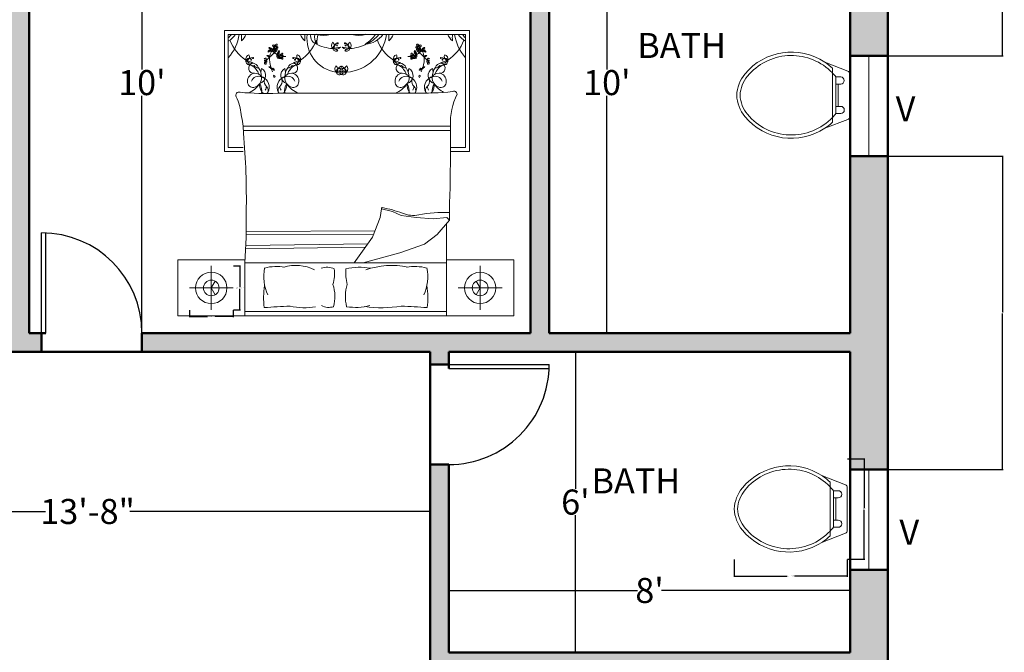
# Model space of a CAD drawing. Units: inches. Extents: x -22 to 470, y -437 to 97.
# Tile 8 of 9: x 235 to 470, y -192 to -41. Entities that reach past the tile are written whole.
import ezdxf

# ---------------------------------------------------------------- set-up
doc = ezdxf.new("R2010")
doc.units = ezdxf.units.IN
doc.header["$MEASUREMENT"] = 0
for name, color, linetype, lineweight in [('A-ANNO-DIMS', 2, 'Continuous', 18), ('A-ANNO-TEXT', 7, 'Continuous', 18), ('A-AREA-IDEN', 7, 'Continuous', 25), ('A-DOOR', 4, 'Continuous', 25), ('A-FLOR-FIXT', 9, 'Continuous', 20), ('A-FURN', 8, 'Continuous', 18), ('A-GLAZ', 4, 'Continuous', 18), ('A-WALL', 7, 'Continuous', 50), ('A-WALL-PATT', 8, 'Continuous', 13)]:
    doc.layers.add(name, color=color, linetype=linetype, lineweight=lineweight)
doc.styles.get("Standard").update_dxf_attribs({"font": 'arial.ttf'})
doc.dimstyles.get("Standard").update_dxf_attribs({"dimtxt": 0.18, "dimasz": 0.18, "dimexe": 0.18, "dimexo": 0.0625, "dimgap": 0.09, "dimtad": 0, "dimtih": 1, "dimtoh": 1, "dimdec": 0, "dimzin": 0, "dimdsep": 46, "dimlunit": 3, "dimtxsty": 'Standard', "dimcen": 0.09, "dimadec": 0, "dimazin": 0, "dimtfac": 1, "dimtdec": 0, "dimtofl": 0, "dimtmove": 0, "dimatfit": 3, "dimfxl": 1, "dimtolj": 1, "dimtzin": 0, "dimarcsym": 0})

# ---------------------------------------------------------------- blocks, each defined once
blk = doc.blocks.new('*D9')
at = {"layer": 'A-ANNO-DIMS', "color": 0, "lineweight": -2, "transparency": 16777216}
for p, q in [((263.92, 4.06), (263.92, -52.6)), ((263.98, 4.24), (264.1, 4.24)), ((263.92, -115.58), (263.92, -58.91)), ((263.98, -115.76), (264.1, -115.76))]:
    blk.add_line(p, q, dxfattribs=at)
at = {"layer": 'A-ANNO-DIMS', "color": 0, "transparency": 16777216}
for points in [[(263.89, 4.06), (263.95, 4.06), (263.92, 4.24)], [(263.89, -115.58), (263.95, -115.58), (263.92, -115.76)]]:
    blk.add_solid(points, dxfattribs=at)
at = {"layer": 'Defpoints', "color": 0, "transparency": 16777216}
for p in [(263.92, 4.24), (263.92, -115.76), (263.92, -115.76)]:
    blk.add_point(p, dxfattribs=at)
at = {"layer": 'A-ANNO-DIMS', "color": 0, "transparency": 16777216, "insert": (263.92, -55.76), "char_height": 6, "attachment_point": 5}
blk.add_mtext("\\A1;10'", dxfattribs=at)
blk = doc.blocks.new('*D11')
at = {"layer": 'A-ANNO-DIMS', "color": 0, "lineweight": -2, "transparency": 16777216}
for p, q in [((386.2, 4.24), (375.02, 4.24)), ((375.2, 4.06), (375.2, -52.6)), ((375.2, -115.58), (375.2, -58.91)), ((386.2, -115.76), (375.02, -115.76))]:
    blk.add_line(p, q, dxfattribs=at)
at = {"layer": 'A-ANNO-DIMS', "color": 0, "transparency": 16777216}
for points in [[(375.17, 4.06), (375.23, 4.06), (375.2, 4.24)], [(375.17, -115.58), (375.23, -115.58), (375.2, -115.76)]]:
    blk.add_solid(points, dxfattribs=at)
at = {"layer": 'Defpoints', "color": 0, "transparency": 16777216}
for p in [(386.26, 4.24), (375.2, -115.76), (386.26, -115.76)]:
    blk.add_point(p, dxfattribs=at)
at = {"layer": 'A-ANNO-DIMS', "color": 0, "transparency": 16777216, "insert": (375.2, -55.76), "char_height": 6, "attachment_point": 5}
blk.add_mtext("\\A1;10'", dxfattribs=at)
blk = doc.blocks.new('*D12')
at = {"layer": 'A-ANNO-DIMS', "color": 0, "lineweight": -2, "transparency": 16777216}
for p, q in [((168.92, -159.44), (168.92, -158.33)), ((169.1, -158.51), (240.81, -158.51)), ((332.74, -158.51), (261.03, -158.51)), ((332.92, -158.44), (332.92, -158.33))]:
    blk.add_line(p, q, dxfattribs=at)
at = {"layer": 'A-ANNO-DIMS', "color": 0, "transparency": 16777216}
for points in [[(169.1, -158.48), (169.1, -158.54), (168.92, -158.51)], [(332.74, -158.48), (332.74, -158.54), (332.92, -158.51)]]:
    blk.add_solid(points, dxfattribs=at)
at = {"layer": 'Defpoints', "color": 0, "transparency": 16777216}
for p in [(168.92, -159.51), (332.92, -158.51), (332.92, -158.51)]:
    blk.add_point(p, dxfattribs=at)
at = {"layer": 'A-ANNO-DIMS', "color": 0, "transparency": 16777216, "insert": (250.92, -158.51), "char_height": 6, "attachment_point": 5}
blk.add_mtext('\\A1;13\'-8"', dxfattribs=at)
blk = doc.blocks.new('*D13')
at = {"layer": 'A-ANNO-DIMS', "color": 0, "lineweight": -2, "transparency": 16777216}
for p, q in [((367.68, -120.44), (367.68, -153.1)), ((367.74, -120.26), (367.86, -120.26)), ((367.68, -192.08), (367.68, -159.41)), ((367.74, -192.26), (367.86, -192.26))]:
    blk.add_line(p, q, dxfattribs=at)
at = {"layer": 'A-ANNO-DIMS', "color": 0, "transparency": 16777216}
for points in [[(367.65, -120.44), (367.71, -120.44), (367.68, -120.26)], [(367.65, -192.08), (367.71, -192.08), (367.68, -192.26)]]:
    blk.add_solid(points, dxfattribs=at)
at = {"layer": 'Defpoints', "color": 0, "transparency": 16777216}
for p in [(367.68, -120.26), (367.68, -192.26), (367.68, -192.26)]:
    blk.add_point(p, dxfattribs=at)
at = {"layer": 'A-ANNO-DIMS', "color": 0, "transparency": 16777216, "insert": (367.68, -156.26), "char_height": 6, "attachment_point": 5}
blk.add_mtext("\\A1;6'", dxfattribs=at)
blk = doc.blocks.new('*D14')
at = {"layer": 'A-ANNO-DIMS', "color": 0, "lineweight": -2, "transparency": 16777216}
for p, q in [((337.42, -175.63), (337.42, -177.62)), ((433.42, -175.63), (433.42, -177.62)), ((337.6, -177.44), (382.57, -177.44)), ((433.24, -177.44), (388.28, -177.44))]:
    blk.add_line(p, q, dxfattribs=at)
at = {"layer": 'A-ANNO-DIMS', "color": 0, "transparency": 16777216}
for points in [[(337.6, -177.41), (337.6, -177.47), (337.42, -177.44)], [(433.24, -177.41), (433.24, -177.47), (433.42, -177.44)]]:
    blk.add_solid(points, dxfattribs=at)
at = {"layer": 'Defpoints', "color": 0, "transparency": 16777216}
for p in [(337.42, -175.57), (433.42, -175.57), (433.42, -177.44)]:
    blk.add_point(p, dxfattribs=at)
at = {"layer": 'A-ANNO-DIMS', "color": 0, "transparency": 16777216, "insert": (385.42, -177.44), "char_height": 6, "attachment_point": 5}
blk.add_mtext("\\A1;8'", dxfattribs=at)
blk = doc.blocks.new('DOOR-SWING-24')
for p, q in [((23, 24), (23, 0)), ((24, 24), (24, 0))]:
    blk.add_line(p, q)
blk.add_arc((24, 24), 24, 180, 270)
blk = doc.blocks.new('WC-PLAN')
for p, q in [((22.94, 16.78), (22.94, 15.64)), ((22.94, 15.64), (22.94, 10.33)), ((22.94, 5.01), (22.94, 10.33)), ((22.94, 5.01), (22.94, 3.87))]:
    blk.add_line(p, q)
for points in [[(21.08, 18.24, 0.383919), (1.95, 15.41, 0.163732), (0, 10.33, 0.359733)], [(22.39, 16.19, 0.431639), (2.57, 14.89, 0.162618), (0.81, 10.33, 0.470877)], [(22.94, 16.78, 0.040937), (21.08, 18.24, 0.163732)], [(27.03, 10.33), (27.03, 15.49, 0.31031), (26.6, 16.12), (21.08, 18.24, 0.209071)], [(22.94, 15.64, 0.014165), (22.39, 16.19, 0.162618)], [(23.75, 14.71, 0.022712), (22.94, 15.64, 0.162618)], [(23.75, 10.33), (23.75, 14.71, 0.022712)], [(23.75, 14.71), (24.89, 14.71, -1), (24.89, 12.99), (24.3, 12.99)], [(21.08, 2.41, -0.383919), (1.95, 5.25, -0.163732), (0, 10.33, -0.359733)], [(22.94, 5.01, -0.448546), (2.57, 5.76, -0.162618), (0.81, 10.33, -0.470877)], [(27.03, 10.33), (27.03, 5.16, -0.31031), (26.6, 4.53), (21.08, 2.41, -0.209071)], [(23.75, 10.33), (23.75, 5.94, -0.476108)], [(23.75, 5.94), (24.89, 5.94, 1), (24.89, 7.67), (24.3, 7.67)], [(23.75, 5.94, -0.022712), (22.94, 5.01, -0.162618)], [(22.94, 3.87, -0.040937), (21.08, 2.41, -0.163732)]]:
    blk.add_lwpolyline(points, format="xyb")
for points in [[(24.3, 12.99), (23.75, 12.99)], [(24.3, 7.67), (24.3, 12.99)], [(24.3, 7.67), (23.75, 7.67)]]:
    blk.add_lwpolyline(points)
blk = doc.blocks.new('BEDSIDE-LAMP-SMALL')
for p, q in [((5.25, 10.51), (5.25, 0)), ((10.51, 5.25), (0, 5.25))]:
    blk.add_line(p, q)
for points in [[(5.25, 5.25), (6.19, 6.88)], [(5.25, 5.25), (6.19, 3.63)]]:
    blk.add_lwpolyline(points)
for radius in [3.75, 1.88]:
    blk.add_circle((5.25, 5.25), radius)
blk = doc.blocks.new('VENT-24-SASH')
for p, q in [((0, 24), (0, 0)), ((4.5, 24), (4.5, 0)), ((9, 0), (9, 24))]:
    blk.add_line(p, q)
blk = doc.blocks.new('*D41')
at = {"layer": 'A-ANNO-DIMS', "color": 0, "lineweight": -2, "transparency": 16777216}
for p, q in [((405.7, -169.98), (405.7, -174.16)), ((432.73, -169.98), (432.73, -174.16)), ((405.88, -173.98), (418.33, -173.98)), ((432.55, -173.98), (420.11, -173.98))]:
    blk.add_line(p, q, dxfattribs=at)
at = {"layer": 'A-ANNO-DIMS', "color": 0, "transparency": 16777216}
for points in [[(405.88, -173.95), (405.88, -174.01), (405.7, -173.98)], [(432.55, -173.95), (432.55, -174.01), (432.73, -173.98)]]:
    blk.add_solid(points, dxfattribs=at)
at = {"layer": 'Defpoints', "color": 0, "transparency": 16777216}
for p in [(405.7, -169.92), (432.73, -169.92), (432.73, -173.98)]:
    blk.add_point(p, dxfattribs=at)
at = {"layer": 'A-ANNO-DIMS', "color": 0, "transparency": 16777216, "insert": (419.22, -173.98), "char_height": 0.18, "attachment_point": 5}
blk.add_mtext('\\A1;WC 2\'-3" TYP.', dxfattribs=at)
blk = doc.blocks.new('*D42')
at = {"layer": 'A-ANNO-DIMS', "color": 0, "lineweight": -2, "transparency": 16777216}
for p, q in [((432.8, -145.91), (436.97, -145.91)), ((436.79, -146.09), (436.79, -157.73)), ((436.79, -169.74), (436.79, -158.1)), ((432.8, -169.92), (436.97, -169.92))]:
    blk.add_line(p, q, dxfattribs=at)
at = {"layer": 'A-ANNO-DIMS', "color": 0, "transparency": 16777216}
for points in [[(436.76, -146.09), (436.82, -146.09), (436.79, -145.91)], [(436.76, -169.74), (436.82, -169.74), (436.79, -169.92)]]:
    blk.add_solid(points, dxfattribs=at)
at = {"layer": 'Defpoints', "color": 0, "transparency": 16777216}
for p in [(432.73, -145.91), (436.79, -145.91), (432.73, -169.92)]:
    blk.add_point(p, dxfattribs=at)
at = {"layer": 'A-ANNO-DIMS', "color": 0, "transparency": 16777216, "insert": (436.79, -157.91), "char_height": 0.18, "attachment_point": 5}
blk.add_mtext('\\A1;2\'-0" TYP.', dxfattribs=at)
blk = doc.blocks.new('*D53')
at = {"layer": 'A-ANNO-DIMS', "color": 0, "lineweight": -2, "transparency": 16777216}
for p, q in [((285.85, -99.7), (287.55, -99.7)), ((287.37, -99.88), (287.37, -104.77)), ((287.37, -110.03), (287.37, -105.14)), ((285.85, -110.21), (287.55, -110.21))]:
    blk.add_line(p, q, dxfattribs=at)
at = {"layer": 'A-ANNO-DIMS', "color": 0, "transparency": 16777216}
for points in [[(287.34, -99.88), (287.4, -99.88), (287.37, -99.7)], [(287.34, -110.03), (287.4, -110.03), (287.37, -110.21)]]:
    blk.add_solid(points, dxfattribs=at)
at = {"layer": 'Defpoints', "color": 0, "transparency": 16777216}
for p in [(285.79, -99.7), (287.37, -99.7), (285.79, -110.21)]:
    blk.add_point(p, dxfattribs=at)
at = {"layer": 'A-ANNO-DIMS', "color": 0, "transparency": 16777216, "insert": (287.37, -104.96), "char_height": 0.18, "attachment_point": 5}
blk.add_mtext('\\A1;LAMP 0\'-10 1/2" TYP.', dxfattribs=at)
blk = doc.blocks.new('*D54')
at = {"layer": 'A-ANNO-DIMS', "color": 0, "lineweight": -2, "transparency": 16777216}
for p, q in [((275.28, -110.27), (275.28, -111.97)), ((285.79, -110.27), (285.79, -111.97)), ((275.46, -111.79), (279.62, -111.79)), ((285.61, -111.79), (281.46, -111.79))]:
    blk.add_line(p, q, dxfattribs=at)
at = {"layer": 'A-ANNO-DIMS', "color": 0, "transparency": 16777216}
for points in [[(275.46, -111.76), (275.46, -111.82), (275.28, -111.79)], [(285.61, -111.76), (285.61, -111.82), (285.79, -111.79)]]:
    blk.add_solid(points, dxfattribs=at)
at = {"layer": 'Defpoints', "color": 0, "transparency": 16777216}
for p in [(275.28, -110.21), (285.79, -110.21), (285.79, -111.79)]:
    blk.add_point(p, dxfattribs=at)
at = {"layer": 'A-ANNO-DIMS', "color": 0, "transparency": 16777216, "insert": (280.54, -111.79), "char_height": 0.18, "attachment_point": 5}
blk.add_mtext('\\A1;0\'-10 1/2" TYP.', dxfattribs=at)
blk = doc.blocks.new('*D70')
at = {"layer": 'A-ANNO-DIMS', "color": 0, "lineweight": -2, "transparency": 16777216}
for p, q in [((442.48, 13.24), (470.05, 13.24)), ((469.87, 13.06), (469.87, -17.88)), ((469.87, -49.2), (469.87, -18.25)), ((442.48, -49.38), (470.05, -49.38))]:
    blk.add_line(p, q, dxfattribs=at)
at = {"layer": 'A-ANNO-DIMS', "color": 0, "transparency": 16777216}
for points in [[(469.84, 13.06), (469.9, 13.06), (469.87, 13.24)], [(469.84, -49.2), (469.9, -49.2), (469.87, -49.38)]]:
    blk.add_solid(points, dxfattribs=at)
at = {"layer": 'Defpoints', "color": 0, "transparency": 16777216}
for p in [(442.42, 13.24), (442.42, -49.38), (469.87, -49.38)]:
    blk.add_point(p, dxfattribs=at)
at = {"layer": 'A-ANNO-DIMS', "color": 0, "transparency": 16777216, "insert": (469.87, -18.07), "char_height": 0.18, "attachment_point": 5}
blk.add_mtext('\\A1;5\'-2 1/2"', dxfattribs=at)
blk = doc.blocks.new('*D71')
at = {"layer": 'A-ANNO-DIMS', "color": 0, "lineweight": -2, "transparency": 16777216}
for p, q in [((442.48, -73.38), (470.05, -73.38)), ((469.87, -73.56), (469.87, -110.75)), ((469.87, -148.31), (469.87, -111.12)), ((442.48, -148.49), (470.05, -148.49))]:
    blk.add_line(p, q, dxfattribs=at)
at = {"layer": 'A-ANNO-DIMS', "color": 0, "transparency": 16777216}
for points in [[(469.84, -73.56), (469.9, -73.56), (469.87, -73.38)], [(469.84, -148.31), (469.9, -148.31), (469.87, -148.49)]]:
    blk.add_solid(points, dxfattribs=at)
at = {"layer": 'Defpoints', "color": 0, "transparency": 16777216}
for p in [(442.42, -73.38), (442.42, -148.49), (469.87, -148.49)]:
    blk.add_point(p, dxfattribs=at)
at = {"layer": 'A-ANNO-DIMS', "color": 0, "transparency": 16777216, "insert": (469.87, -110.94), "char_height": 0.18, "attachment_point": 5}
blk.add_mtext('\\A1;6\'-3"', dxfattribs=at)

msp = doc.modelspace()

# ---------------------------------------------------------------- hatches: boundary and pattern name
at = {"layer": 'A-WALL-PATT'}
h = msp.add_hatch(color=256, dxfattribs=at)
h.dxf.hatch_style = 1
h.paths.add_polyline_path([(130.42, 13.24), (26.92, 13.24), (26.92, -43.76), (35.92, -43.76), (35.92, 4.24), (83.92, 4.24), (83.92, 1.24), (88.42, 1.24), (88.42, 4.24), (130.42, 4.24)])
h.paths.add_polyline_path([(266.92, 13.24), (190.42, 13.24), (190.42, 4.24), (232.42, 4.24), (232.42, -115.76), (229.42, -115.76), (229.42, -120.26), (239.92, -120.26), (239.92, -115.76), (236.92, -115.76), (236.92, 4.24), (266.92, 4.24)])
h.paths.add_polyline_path([(442.42, 13.24), (326.92, 13.24), (326.92, 4.24), (356.92, 4.24), (356.92, 1.24), (361.42, 1.24), (361.42, 4.24), (433.42, 4.24), (433.42, -49.38), (442.42, -49.38)])
h.paths.add_polyline_path([(442.42, -73.38), (433.42, -73.38), (433.42, -115.76), (361.42, -115.76), (361.42, -22.76), (356.92, -22.76), (356.92, -115.76), (263.92, -115.76), (263.92, -120.26), (332.92, -120.26), (332.92, -123.26), (337.42, -123.26), (337.42, -120.26), (433.42, -120.26), (433.42, -148.49), (442.42, -148.49)])
h.paths.add_polyline_path([(205.42, -115.76), (88.42, -115.76), (88.42, -22.76), (83.92, -22.76), (83.92, -115.76), (35.92, -115.76), (35.92, -67.76), (26.92, -67.76), (26.92, -126.26), (35.92, -126.26), (35.92, -120.26), (205.42, -120.26)])
h.paths.add_polyline_path([(35.92, -196.76), (168.92, -196.76), (168.92, -192.26), (35.92, -192.26), (35.92, -186.26), (26.92, -186.26), (26.92, -224.25), (35.92, -224.25)])
h.paths.add_polyline_path([(35.92, -284.25), (26.92, -284.25), (26.92, -397.76), (53.92, -397.76), (53.92, -388.76), (35.92, -388.76)])
h.paths.add_polyline_path([(142.42, -388.76), (136.42, -388.76), (136.42, -316.76), (181.42, -316.76), (181.42, -312.26), (136.42, -312.26), (136.42, -303.75), (131.92, -303.75), (131.92, -388.76), (113.92, -388.76), (113.92, -397.76), (142.42, -397.76)])
h.paths.add_polyline_path([(218.92, -388.76), (212.92, -388.76), (212.92, -312.26), (205.42, -312.26), (205.42, -316.76), (208.42, -316.76), (208.42, -388.76), (202.42, -388.76), (202.42, -397.76), (218.92, -397.76)])
h.paths.add_polyline_path([(306.75, -388.76), (289.42, -388.76), (289.42, -316.76), (284.92, -316.76), (284.92, -388.76), (278.92, -388.76), (278.92, -397.76), (306.75, -397.76)])
h.paths.add_polyline_path([(391.42, -388.76), (366.75, -388.76), (366.75, -397.76), (391.42, -397.76)], flags=17)
h.paths.add_polyline_path([(442.42, -172.49), (433.42, -172.49), (433.42, -192.26), (337.42, -192.26), (337.42, -147.26), (332.92, -147.26), (332.92, -196.76), (433.42, -196.76), (433.42, -388.76), (427.42, -388.76), (427.42, -397.76), (442.42, -397.76)])

# ---------------------------------------------------------------- linework, layer by layer
at = {"layer": 'A-FURN'}
for p, q in [((283.67, -43.27), (342.3, -43.27)), ((283.67, -72.24), (283.67, -43.27)), ((284.6, -44.2), (284.6, -71.31)), ((341.37, -44.2), (284.6, -44.2)), ((341.37, -71.31), (341.37, -44.2)), ((342.3, -43.27), (342.3, -72.24)), ((292.53, -52.35), (292.35, -53.26)), ((298.15, -52.35), (298.33, -53.26)), ((327.82, -52.35), (327.64, -53.26)), ((333.44, -52.35), (333.62, -53.26)), ((296.38, -58.32), (329.03, -58.32)), ((288.14, -66.22), (337.76, -66.22)), ((288.21, -67.22), (337.76, -67.22)), ((288.13, -72.24), (283.67, -72.24)), ((284.6, -71.31), (288.15, -71.31)), ((337.75, -71.31), (341.37, -71.31)), ((342.3, -72.24), (337.75, -72.24)), ((320.94, -88.1), (321.26, -85.98)), ((321.26, -85.98), (323.87, -86.63)), ((323.87, -86.63), (325.99, -87.61)), ((319.14, -92.82), (320.94, -88.1)), ((325.99, -87.61), (329.57, -88.1)), ((329.57, -88.1), (333.64, -88.42)), ((333.64, -88.42), (336.9, -88.1)), ((337.55, -88.75), (334.62, -92.17)), ((336.9, -88.1), (337.55, -88.75)), ((288.86, -91.43), (319.72, -91.3)), ((336.83, -111.66), (336.83, -89.59)), ((288.87, -92.25), (319.4, -92.13)), ((314.74, -98.95), (319.14, -92.82)), ((334.62, -92.17), (331.52, -94.44)), ((288.8, -95.61), (317.43, -95.21)), ((288.83, -94.78), (318.03, -94.37)), ((325.66, -96.56), (316.89, -98.95)), ((331.52, -94.44), (325.66, -96.56)), ((336.83, -98.95), (288.58, -98.95)), ((288.58, -110.63), (336.83, -110.63)), ((352.91, -111.66), (272.5, -111.66))]:
    msp.add_line(p, q, dxfattribs=at)
for points in [[(337.72, -81.38, 0.001242), (337.76, -66.13, -0.127202), (339.37, -58.52)], [(288.24, -67.86, 0.056112), (287.65, -63.43, 0.095341), (286.52, -59.17)], [(293.2, -109.65, -0.074897), (293.3, -104.4, 0.472817)], [(309.65, -104.11, -0.14099), (309.81, -109.47, -0.235245)], [(313.08, -104.11, 0.14099), (312.92, -109.47, 0.235245)], [(332.21, -109.65, 0.074897), (332.11, -104.4, -0.472817)]]:
    msp.add_lwpolyline(points, format="xyb", dxfattribs=at)
for points in [[(288.58, -111.66), (288.58, -98.26), (272.5, -98.26), (272.5, -111.66)], [(336.83, -98.26), (352.91, -98.26), (352.91, -111.66)]]:
    msp.add_lwpolyline(points, dxfattribs=at)
for centre in [(295.83, -47.28), (330.14, -47.28), (297.17, -49.44), (328.8, -49.44)]:
    msp.add_circle(centre, 0.205, dxfattribs=at)
for centre, radius, start, end in [((282.05, -41.38), 5.12, 299.8884, 326.5383), ((280.21, -40.43), 6.38, 313.5186, 323.6964), ((276.79, -42.79), 10.5, 318.1144, 352.255), ((284.92, -42.56), 4.27, 311.0454, 337.4453), ((273.22, -44.86), 14.53, 356.3481, 2.5919), ((305.76, -42.56), 4.27, 202.5547, 228.9546), ((317.45, -44.86), 14.53, 177.4081, 183.6519), ((311.55, -45.21), 8.13, 172.8636, 261.8197), ((306.19, -44.65), 1.88, 166.3898, 259.0739), ((307.6, -44.9), 2.38, 162.8609, 221.9049), ((307.47, -38.68), 5.77, 252.9798, 286.4569), ((310.5, -45.95), 4.7, 158.117, 186.6195), ((309.76, -35.7), 8.54, 264.3643, 265.6213), ((314.25, -29.85), 15.26, 250.0972, 250.2783), ((312.08, -42.79), 10.5, 274.4623, 352.255), ((315.82, -38.68), 5.77, 253.5431, 287.0202), ((313.53, -35.7), 8.54, 274.3787, 275.6357), ((309.04, -29.85), 15.26, 289.7217, 289.9028), ((317.35, -41.38), 5.12, 271.272, 326.5383), ((312.16, -38.63), 9.49, 304.0123, 324.053), ((315.51, -40.43), 6.38, 287.8504, 323.6964), ((308.52, -44.86), 14.53, 356.3481, 2.5919), ((320.21, -42.56), 4.27, 311.0454, 337.4453), ((341.05, -42.56), 4.27, 202.5547, 228.9546), ((352.75, -44.86), 14.53, 177.4081, 183.6519), ((349.18, -42.79), 10.5, 187.745, 221.8856), ((343.92, -41.38), 5.12, 213.4617, 240.1116), ((345.76, -40.43), 6.38, 216.3036, 226.4814), ((294.75, -41.75), 10.5, 201.4092, 235.6135), ((295.4, -46.9), 0.203, 134.3732, 211.9501), ((295.78, -46.66), 0.646, 211.9501, 255.2442), ((295.42, -47.13), 0.404, 8.5614, 112.5914), ((295.53, -47.11), 0.136, 352.868, 97.094), ((296.11, -46.9), 0.338, 100.9597, 208.7804), ((296.48, -47.35), 0.622, 132.3896, 156.5724), ((296.21, -47.43), 0.335, 42.3208, 130.2111), ((295.83, -46.72), 0.476, 291.6382, 4.947), ((296.15, -46.7), 0.157, 4.947, 127.5263), ((295.93, -41.75), 10.5, 304.3865, 338.5908), ((310.41, -37.16), 10.5, 242.5854, 265.5377), ((310.45, -46.85), 1.16, 140.8855, 222.2127), ((309.13, -46.88), 0.877, 301.6373, 61.4609), ((312.1, -48.49), 2.66, 121.989, 161.0841), ((310.45, -47.6), 0.859, 76.148, 182.2415), ((310.64, -46.92), 0.0685, 140.1909, 76.0209), ((310.76, -46.35), 0.13, 288.4408, 121.989), ((310.79, -46.41), 0.0634, 171.9833, 288.4408), ((312.53, -46.35), 0.13, 58.011, 251.5592), ((312.5, -46.41), 0.0634, 251.5592, 8.0167), ((312.66, -46.87), 0.114, 103.852, 39.9245), ((311.19, -48.49), 2.66, 18.9159, 58.011), ((312.84, -47.6), 0.859, 357.7585, 103.852), ((314.16, -46.88), 0.877, 118.5391, 238.3627), ((312.84, -46.85), 1.16, 317.7873, 39.1145), ((312.88, -37.16), 10.5, 274.4623, 297.4146), ((330.05, -41.75), 10.5, 201.4092, 235.6135), ((329.77, -47.43), 0.335, 49.7889, 137.6792), ((329.83, -46.7), 0.157, 52.4737, 175.053), ((330.14, -46.72), 0.476, 175.053, 248.3618), ((329.49, -47.35), 0.622, 23.4276, 47.6104), ((329.86, -46.9), 0.338, 331.2196, 79.0403), ((330.55, -47.13), 0.404, 67.4086, 171.4386), ((330.44, -47.11), 0.136, 82.906, 187.132), ((330.19, -46.66), 0.646, 284.7558, 328.0499), ((330.57, -46.9), 0.203, 328.0499, 45.6268), ((331.22, -41.75), 10.5, 304.3865, 338.5908), ((289.96, -50.17), 1.16, 110.9613, 192.2885), ((288.79, -49.54), 0.877, 271.7131, 31.5367), ((293.89, -51.52), 2.27, 82.8698, 91.6736), ((294.2, -49.07), 0.422, 205.5379, 258.6744), ((293.59, -50.5), 1.27, 59.344, 79.7412), ((294.34, -48.33), 0.229, 123.0979, 213.1364), ((293.32, -50.5), 1.29, 43.6929, 51.7899), ((294.74, -48.66), 0.619, 92.3172, 160.5201), ((297.57, -53.37), 5.98, 121.1156, 124.8118), ((294.11, -49.65), 0.386, 355.7131, 81.6568), ((294.67, -48.43), 0.533, 82.6008, 147.1845), ((293.9, -49.99), 0.674, 27.3659, 59.344), ((294.51, -47.58), 0.229, 55.6077, 145.6462), ((294.36, -48.07), 0.619, 21.7087, 93.0299), ((291.09, -52.49), 5.98, 53.6254, 57.3216), ((294.6, -48.45), 0.237, 45.7354, 121.1156), ((297.83, -49.96), 3.34, 150.7959, 175.244), ((302.63, -57.07), 10.99, 127.8256, 137.7588), ((294.55, -47.92), 0.533, 342.8042, 79.6943), ((294.5, -47.86), 0.237, 338.2452, 53.6254), ((294.89, -48.01), 0.179, 158.2452, 340.6395), ((294.89, -48.15), 0.179, 225.7354, 48.1297), ((298.25, -46.52), 3.57, 201.7087, 206.2181), ((295.41, -48.96), 0.933, 40.9365, 112.7695), ((295.1, -48.64), 0.549, 49.3812, 95.5456), ((297.83, -49.96), 3.34, 137.5083, 145.9967), ((295.5, -48.43), 0.567, 61.1838, 141.6792), ((298.17, -45.52), 4.01, 220.182, 239.456), ((295.61, -47.57), 0.279, 88.5719, 233.8954), ((295.58, -47.64), 0.201, 228.2946, 6.2474), ((295.89, -47.73), 0.66, 229.3812, 289.9959), ((295.39, -47.4), 0.282, 298.8493, 359.9355), ((295.46, -47.64), 0.322, 4.2123, 48.1587), ((296.12, -47.6), 0.342, 183.635, 258.4363), ((295.46, -48.53), 0.678, 15.6484, 62.2957), ((296.07, -47.48), 0.196, 178.1325, 268.8919), ((296.28, -47.08), 0.423, 226.3462, 279.6513), ((295.84, -47.87), 0.492, 7.4968, 71.2737), ((296.2, -46.64), 0.67, 254.2829, 276.9148), ((296.18, -47.84), 0.158, 215.0752, 14.7644), ((296.11, -49.54), 0.567, 3.8774, 87.1501), ((295.85, -48.09), 0.933, 287.889, 359.722), ((295.82, -48.53), 0.549, 305.1128, 351.2773), ((295.7, -49.32), 0.549, 352.0748, 38.2393), ((295.61, -49.75), 0.933, 343.6301, 55.4631), ((296.9, -49.48), 0.66, 172.0748, 232.6895), ((296.27, -48.43), 0.567, 271.4625, 339.4747), ((296.32, -47.33), 0.176, 279.6513, 42.3208), ((297.02, -48.71), 0.66, 110.6625, 171.2773), ((296.74, -49.06), 0.203, 134.3732, 211.9501), ((298.17, -45.52), 4.01, 246.1523, 246.9499), ((297.12, -48.82), 0.646, 211.9501, 255.2442), ((296.76, -49.28), 0.404, 8.5614, 112.5914), ((296.95, -49.73), 0.279, 88.5719, 233.8954), ((296.17, -48.38), 0.678, 338.3627, 25.0101), ((296.87, -49.27), 0.136, 352.868, 97.094), ((297.45, -49.06), 0.338, 100.9597, 208.7804), ((297.82, -49.51), 0.622, 132.3896, 156.5724), ((297.54, -49.59), 0.335, 42.3208, 130.2111), ((297.17, -48.88), 0.476, 291.6382, 4.947), ((297.54, -48.8), 0.67, 254.2829, 276.9148), ((297.48, -48.85), 0.157, 4.947, 127.5263), ((297.66, -49.48), 0.176, 279.6513, 42.3208), ((301.88, -49.54), 0.877, 148.4633, 268.2869), ((300.72, -50.17), 1.16, 347.7115, 69.0387), ((311.79, -54.64), 7.35, 92.7418, 107.407), ((310.27, -46.12), 1.66, 245.6899, 314.4589), ((309.54, -49.42), 1.79, 44.6273, 88.5415), ((310.43, -47.39), 0.871, 196.1963, 296.9726), ((311.5, -54.64), 7.35, 72.593, 87.2582), ((313.02, -46.12), 1.66, 225.5411, 294.3101), ((313.75, -49.42), 1.79, 91.4585, 135.3727), ((312.86, -47.39), 0.871, 243.0274, 343.8037), ((325.25, -50.17), 1.16, 110.9613, 192.2885), ((324.09, -49.54), 0.877, 271.7131, 31.5367), ((328.31, -49.48), 0.176, 137.6792, 260.3487), ((328.43, -49.59), 0.335, 49.7889, 137.6792), ((328.49, -48.85), 0.157, 52.4737, 175.053), ((328.8, -48.88), 0.476, 175.053, 248.3618), ((328.43, -48.8), 0.67, 263.0852, 285.7171), ((328.15, -49.51), 0.622, 23.4276, 47.6104), ((328.52, -49.06), 0.338, 331.2196, 79.0403), ((329.21, -49.28), 0.404, 67.4086, 171.4386), ((329.1, -49.27), 0.136, 82.906, 187.132), ((328.85, -48.82), 0.646, 284.7558, 328.0499), ((329.02, -49.73), 0.279, 306.1046, 91.4281), ((329.8, -48.38), 0.678, 154.9899, 201.6373), ((329.7, -48.43), 0.567, 200.5253, 268.5375), ((330.12, -48.09), 0.933, 180.278, 252.111), ((328.96, -48.71), 0.66, 8.7227, 69.3375), ((329.87, -49.54), 0.567, 92.8499, 176.1226), ((329.23, -49.06), 0.203, 328.0499, 45.6268), ((327.8, -45.52), 4.01, 293.0501, 293.8477), ((330.36, -49.75), 0.933, 124.5369, 196.3699), ((329.65, -47.33), 0.176, 137.6792, 260.3487), ((329.07, -49.48), 0.66, 307.3105, 7.9252), ((330.15, -48.53), 0.549, 188.7227, 234.8872), ((329.69, -47.08), 0.423, 260.3487, 313.6538), ((329.79, -47.84), 0.158, 165.2356, 324.9248), ((330.13, -47.87), 0.492, 108.7263, 172.5032), ((329.77, -46.64), 0.67, 263.0852, 285.7171), ((330.27, -49.32), 0.549, 141.7607, 187.9252), ((327.8, -45.52), 4.01, 300.544, 319.818), ((330.51, -48.53), 0.678, 117.7043, 164.3516), ((330.56, -48.96), 0.933, 67.2305, 139.0635), ((330.08, -47.73), 0.66, 250.0041, 310.6188), ((329.9, -47.48), 0.196, 271.1081, 1.8675), ((329.85, -47.6), 0.342, 281.5637, 356.365), ((323.34, -57.07), 10.99, 42.2412, 52.1744), ((330.51, -47.64), 0.322, 131.8413, 175.7877), ((330.39, -47.64), 0.201, 173.7526, 311.7054), ((330.47, -48.43), 0.567, 38.3208, 118.8162), ((330.58, -47.4), 0.282, 180.0645, 241.1507), ((330.36, -47.57), 0.279, 306.1046, 91.4281), ((330.87, -48.64), 0.549, 84.4544, 130.6188), ((328.15, -49.96), 3.34, 34.0033, 42.4917), ((331.42, -47.92), 0.533, 100.3057, 197.1958), ((331.08, -48.15), 0.179, 131.8703, 314.2646), ((331.08, -48.01), 0.179, 199.3605, 21.7548), ((327.72, -46.52), 3.57, 333.7819, 338.2913), ((331.61, -48.07), 0.619, 86.9701, 158.2913), ((328.15, -49.96), 3.34, 4.756, 29.2041), ((331.37, -48.45), 0.237, 58.8844, 134.2646), ((331.47, -47.86), 0.237, 126.3746, 201.7548), ((331.3, -48.43), 0.533, 32.8155, 97.3992), ((331.23, -48.66), 0.619, 19.4799, 87.6828), ((331.46, -47.58), 0.229, 34.3538, 124.3923), ((334.88, -52.49), 5.98, 122.6784, 126.3746), ((331.86, -49.65), 0.386, 98.3432, 184.2869), ((332.07, -49.99), 0.674, 120.656, 152.6341), ((328.4, -53.37), 5.98, 55.1882, 58.8844), ((332.65, -50.5), 1.29, 128.2101, 136.3071), ((332.38, -50.5), 1.27, 100.2588, 120.656), ((331.63, -48.33), 0.229, 326.8636, 56.9021), ((332.08, -51.52), 2.27, 88.3264, 97.1302), ((331.77, -49.07), 0.422, 281.3256, 334.4621), ((337.18, -49.54), 0.877, 148.4633, 268.2869), ((336.01, -50.17), 1.16, 347.7115, 69.0387), ((289.67, -50.62), 0.871, 166.272, 267.0484), ((290.57, -52.41), 2.66, 92.0648, 131.1598), ((289.58, -50.81), 0.859, 46.2238, 152.3173), ((287.23, -57.59), 7.35, 62.8176, 77.4827), ((290.17, -49.44), 1.66, 215.7657, 284.5347), ((287.89, -51.95), 1.79, 14.7031, 58.6173), ((290.69, -52.29), 1.21, 109.1312, 279.736), ((290.44, -50.98), 0.74, 216.7319, 296.0245), ((290.08, -50.32), 0.0685, 110.2667, 46.2271), ((288.3, -54.95), 3.8, 18.2955, 58.7386), ((290.4, -52.65), 1.51, 15.6955, 94.031), ((290.46, -49.96), 0.0634, 142.0591, 258.5166), ((290.48, -49.89), 0.13, 258.5166, 92.0648), ((292.02, -50.65), 1.61, 218.4175, 263.8338), ((293.48, -50.28), 0.338, 100.9597, 142.2379), ((293.2, -50.66), 0.205, 273.2768, 86.7232), ((293.49, -50.98), 0.342, 217.3642, 258.4363), ((293.44, -50.85), 0.196, 178.1325, 268.8919), ((293.85, -50.73), 0.622, 132.3896, 156.5724), ((293.57, -50.81), 0.335, 42.3208, 130.2111), ((293.65, -50.46), 0.423, 226.3462, 279.6513), ((293.2, -50.1), 0.476, 291.6382, 4.947), ((293.21, -51.24), 0.492, 7.4968, 71.2737), ((293.57, -50.02), 0.67, 254.2829, 276.9148), ((293.51, -50.07), 0.157, 4.947, 127.5263), ((293.55, -51.22), 0.158, 215.0752, 14.7644), ((288.93, -44.46), 7.64, 307.9541, 316.8459), ((293.69, -50.7), 0.176, 279.6513, 42.3208), ((294.41, -49.54), 0.164, 202.5583, 304.2343), ((301.14, -50.12), 6.66, 176.1723, 196.4158), ((296, -49.56), 0.678, 318.342, 4.9894), ((296.92, -49.8), 0.201, 228.2946, 6.2474), ((296.73, -49.56), 0.282, 298.8493, 359.9355), ((296.8, -49.8), 0.322, 4.2123, 48.1587), ((297.46, -49.76), 0.342, 183.635, 258.4363), ((297.41, -49.63), 0.196, 178.1325, 268.8919), ((297.62, -49.24), 0.423, 226.3462, 279.6513), ((297.18, -50.03), 0.492, 7.4968, 71.2737), ((297.52, -50), 0.158, 215.0752, 14.7644), ((298.17, -45.52), 4.01, 265.2415, 272.8929), ((302.38, -54.95), 3.8, 121.2614, 161.7045), ((300.28, -52.65), 1.51, 85.969, 164.3045), ((298.65, -50.65), 1.61, 276.1662, 321.5825), ((299.99, -52.29), 1.21, 260.264, 70.8688), ((300.24, -50.98), 0.74, 243.9755, 323.2681), ((300.2, -49.89), 0.13, 87.9352, 281.4834), ((300.51, -49.44), 1.66, 255.4653, 324.2343), ((303.45, -57.59), 7.35, 102.5173, 117.1824), ((300.11, -52.41), 2.66, 48.8402, 87.9352), ((300.21, -49.96), 0.0634, 281.4834, 37.9409), ((300.58, -50.28), 0.114, 133.7762, 69.7183), ((301.1, -50.81), 0.859, 27.6827, 133.7762), ((301.01, -50.62), 0.871, 272.9516, 13.728), ((302.79, -51.95), 1.79, 121.3827, 165.2969), ((311.26, -52.47), 1.16, 140.8855, 222.2127), ((309.93, -52.51), 0.877, 301.6373, 61.4609), ((311.57, -51.98), 0.13, 288.4408, 121.989), ((311.72, -51.98), 0.13, 58.011, 251.5592), ((313.36, -52.51), 0.877, 118.5391, 238.3627), ((312.03, -52.47), 1.16, 317.7873, 39.1145), ((324.96, -50.62), 0.871, 166.272, 267.0484), ((325.86, -52.41), 2.66, 92.0648, 131.1598), ((324.88, -50.81), 0.859, 46.2238, 152.3173), ((323.18, -51.95), 1.79, 14.7031, 58.6173), ((325.46, -49.44), 1.66, 215.7657, 284.5347), ((322.52, -57.59), 7.35, 62.8176, 77.4827), ((325.98, -52.29), 1.21, 109.1312, 279.736), ((325.73, -50.98), 0.74, 216.7319, 296.0245), ((325.38, -50.32), 0.0685, 110.2667, 46.2271), ((323.59, -54.95), 3.8, 18.2955, 58.7386), ((325.69, -52.65), 1.51, 15.6955, 94.031), ((325.76, -49.96), 0.0634, 142.0591, 258.5166), ((325.77, -49.89), 0.13, 258.5166, 92.0648), ((327.32, -50.65), 1.61, 218.4175, 263.8338), ((327.8, -45.52), 4.01, 267.1071, 274.7585), ((328.35, -49.24), 0.423, 260.3487, 313.6538), ((328.45, -50), 0.158, 165.2356, 324.9248), ((328.79, -50.03), 0.492, 108.7263, 172.5032), ((328.56, -49.63), 0.196, 271.1081, 1.8675), ((328.51, -49.76), 0.342, 281.5637, 356.365), ((329.18, -49.8), 0.322, 131.8413, 175.7877), ((329.05, -49.8), 0.201, 173.7526, 311.7054), ((329.24, -49.56), 0.282, 180.0645, 241.1507), ((329.98, -49.56), 0.678, 175.0106, 221.658), ((324.83, -50.12), 6.66, 343.5842, 3.8277), ((331.57, -49.54), 0.164, 235.7657, 337.4417), ((337.04, -44.46), 7.64, 223.1541, 232.0459), ((332.28, -50.7), 0.176, 137.6792, 260.3487), ((332.4, -50.81), 0.335, 49.7889, 137.6792), ((332.32, -50.46), 0.423, 260.3487, 313.6538), ((332.42, -51.22), 0.158, 165.2356, 324.9248), ((332.76, -51.24), 0.492, 108.7263, 172.5032), ((332.46, -50.07), 0.157, 52.4737, 175.053), ((332.77, -50.1), 0.476, 175.053, 248.3618), ((332.4, -50.02), 0.67, 263.0852, 285.7171), ((332.53, -50.85), 0.196, 271.1081, 1.8675), ((332.12, -50.73), 0.622, 23.4276, 47.6104), ((332.49, -50.28), 0.338, 37.7621, 79.0403), ((332.48, -50.98), 0.342, 281.5637, 322.6358), ((332.77, -50.66), 0.205, 93.2768, 266.7232), ((337.67, -54.95), 3.8, 121.2614, 161.7045), ((335.57, -52.65), 1.51, 85.969, 164.3045), ((333.95, -50.65), 1.61, 276.1662, 321.5825), ((335.28, -52.29), 1.21, 260.264, 70.8688), ((335.53, -50.98), 0.74, 243.9755, 323.2681), ((335.49, -49.89), 0.13, 87.9352, 281.4834), ((338.74, -57.59), 7.35, 102.5173, 117.1824), ((335.8, -49.44), 1.66, 255.4653, 324.2343), ((335.4, -52.41), 2.66, 48.8402, 87.9352), ((335.51, -49.96), 0.0634, 281.4834, 37.9409), ((335.87, -50.28), 0.114, 133.7762, 69.7183), ((336.39, -50.81), 0.859, 27.6827, 133.7762), ((338.08, -51.95), 1.79, 121.3827, 165.2969), ((336.3, -50.62), 0.871, 272.9516, 13.728), ((291.13, -55.39), 1.92, 97.1143, 185.0551), ((290.8, -55.81), 2.34, 35.9599, 87.6409), ((288.26, -54.64), 4.32, 3.4924, 33.7117), ((291.53, -54.09), 2, 286.8663, 60.0915), ((294.37, -54.22), 2.27, 82.8698, 91.6736), ((294.68, -51.78), 0.422, 205.5379, 258.6744), ((294.07, -53.21), 1.27, 59.344, 79.7412), ((293.8, -53.2), 1.29, 43.6929, 51.7899), ((294.59, -52.36), 0.386, 355.7131, 81.6568), ((294.38, -52.69), 0.674, 27.3659, 59.344), ((294.88, -52.25), 0.164, 202.5583, 304.2343), ((301.14, -50.12), 6.66, 200.1059, 206.9968), ((295.18, -52.71), 0.386, 36.5232, 122.4668), ((294.99, -53.06), 0.674, 58.836, 90.8141), ((295.14, -52.4), 0.164, 173.9457, 275.6216), ((294.81, -53.81), 1.29, 66.3901, 74.4871), ((295.65, -52.36), 0.422, 219.5056, 272.6421), ((294.68, -53.57), 1.27, 38.4388, 58.836), ((295.57, -54.17), 0.155, 79.5616, 257.2949), ((293.64, -53.79), 2.27, 26.5064, 35.3102), ((295.55, -54.27), 0.252, 259.5864, 79.5616), ((299.15, -54.09), 2, 119.9085, 253.1337), ((299.88, -55.81), 2.34, 92.3591, 144.0401), ((302.42, -54.64), 4.32, 146.2883, 176.5076), ((299.55, -55.39), 1.92, 354.9449, 82.8857), ((312.91, -54.12), 2.66, 121.989, 161.0841), ((311.25, -53.22), 0.859, 76.148, 182.2415), ((311.08, -51.74), 1.66, 245.6899, 314.4589), ((312.59, -60.27), 7.35, 92.7418, 107.407), ((311.23, -53.01), 0.871, 196.1963, 296.9726), ((310.35, -55.05), 1.79, 44.6273, 88.5415), ((312.21, -51.74), 1.66, 225.5411, 294.3101), ((310.7, -60.27), 7.35, 72.593, 87.2582), ((311.44, -52.54), 0.0685, 140.1909, 76.0209), ((311.59, -52.04), 0.0634, 171.9833, 288.4408), ((312.06, -53.01), 0.871, 243.0274, 343.8037), ((312.94, -55.05), 1.79, 91.4585, 135.3727), ((311.7, -52.04), 0.0634, 251.5592, 8.0167), ((311.86, -52.5), 0.114, 103.852, 39.9245), ((310.38, -54.12), 2.66, 18.9159, 58.011), ((312.04, -53.22), 0.859, 357.7585, 103.852), ((326.42, -55.39), 1.92, 97.1143, 185.0551), ((326.09, -55.81), 2.34, 35.9599, 87.6409), ((323.55, -54.64), 4.32, 3.4924, 33.7117), ((326.83, -54.09), 2, 286.8663, 60.0915), ((330.42, -54.27), 0.252, 100.4384, 280.4136), ((331.29, -53.57), 1.27, 121.164, 141.5612), ((332.33, -53.79), 2.27, 144.6898, 153.4936), ((330.32, -52.36), 0.422, 267.3579, 320.4944), ((330.4, -54.17), 0.155, 282.7051, 100.4384), ((330.79, -52.71), 0.386, 57.5332, 143.4768), ((330.98, -53.06), 0.674, 89.1859, 121.164), ((331.16, -53.81), 1.29, 105.5129, 113.6099), ((324.83, -50.12), 6.66, 333.0032, 339.8941), ((330.83, -52.4), 0.164, 264.3784, 6.0543), ((331.38, -52.36), 0.386, 98.3432, 184.2869), ((331.59, -52.69), 0.674, 120.656, 152.6341), ((331.09, -52.25), 0.164, 235.7657, 337.4417), ((332.17, -53.2), 1.29, 128.2101, 136.3071), ((331.9, -53.21), 1.27, 100.2588, 120.656), ((331.6, -54.22), 2.27, 88.3264, 97.1302), ((331.29, -51.78), 0.422, 281.3256, 334.4621), ((334.44, -54.09), 2, 119.9085, 253.1337), ((335.17, -55.81), 2.34, 92.3591, 144.0401), ((337.71, -54.64), 4.32, 146.2883, 176.5076), ((334.84, -55.39), 1.92, 354.9449, 82.8857), ((290.57, -55.58), 1.36, 178.9462, 275.5144), ((287.03, -52.66), 6.09, 293.6453, 326.3329), ((291.89, -56.11), 1.87, 68.5779, 158.4181), ((290.16, -54.58), 2.42, 283.079, 4.7067), ((295.19, -56.28), 3.1, 175.2696, 214.215), ((289.26, -57.73), 3.33, 349.249, 31.1782), ((295.19, -56.28), 3.1, 143.6555, 147.2989), ((292.8, -54.93), 0.499, 344.8529, 102.6959), ((291.84, -56.86), 2.56, 330.8249, 70.7178), ((294.87, -55.49), 1.65, 164.8529, 228.4347), ((298.84, -56.86), 2.56, 109.2822, 209.1751), ((295.81, -55.49), 1.65, 311.5653, 15.1471), ((297.88, -54.93), 0.499, 77.3041, 195.1471), ((295.49, -56.28), 3.1, 32.7011, 36.3445), ((295.49, -56.28), 3.1, 325.785, 4.7304), ((301.42, -57.73), 3.33, 148.8218, 190.2867), ((300.52, -54.58), 2.42, 175.2933, 256.921), ((298.79, -56.11), 1.87, 21.5819, 111.4221), ((303.65, -52.66), 6.09, 213.6671, 248.5059), ((300.1, -55.58), 1.36, 264.4856, 1.0538), ((325.87, -55.58), 1.36, 178.9462, 275.5144), ((322.32, -52.66), 6.09, 291.4941, 326.3329), ((327.18, -56.11), 1.87, 68.5779, 158.4181), ((325.45, -54.58), 2.42, 283.079, 4.7067), ((330.48, -56.28), 3.1, 175.2696, 214.215), ((324.55, -57.73), 3.33, 349.7133, 31.1782), ((330.48, -56.28), 3.1, 143.6555, 147.2989), ((328.09, -54.93), 0.499, 344.8529, 102.6959), ((327.14, -56.86), 2.56, 330.8249, 70.7178), ((330.16, -55.49), 1.65, 164.8529, 228.4347), ((334.13, -56.86), 2.56, 109.2822, 209.1751), ((331.1, -55.49), 1.65, 311.5653, 15.1471), ((333.17, -54.93), 0.499, 77.3041, 195.1471), ((330.78, -56.28), 3.1, 32.7011, 36.3445), ((330.78, -56.28), 3.1, 325.785, 4.7304), ((336.71, -57.73), 3.33, 148.8218, 189.1554), ((335.81, -54.58), 2.42, 175.2933, 256.921), ((334.08, -56.11), 1.87, 21.5819, 111.4221), ((338.94, -52.66), 6.09, 213.6671, 243.2997), ((335.4, -55.58), 1.36, 264.4856, 1.0538), ((287.13, -58.76), 0.733, 66.5219, 213.8264), ((293.92, 19.89), 78.25, 265.2402, 271.8035), ((293.39, -57.43), 0.968, 217.675, 252.5814), ((291.45, -56.4), 2.31, 330.0851, 352.564), ((293.39, -57.43), 0.968, 286.6343, 315.5483), ((292.98, -57.62), 1.2, 336.1646, 48.4347), ((297.7, -57.62), 1.2, 131.5653, 203.8354), ((297.29, -57.43), 0.968, 224.4517, 246.7144), ((299.22, -56.4), 2.31, 187.436, 209.9149), ((297.29, -57.43), 0.968, 293.2856, 322.325), ((328.68, -57.43), 0.968, 217.675, 246.7144), ((326.75, -56.4), 2.31, 330.0851, 352.564), ((329.99, 25.39), 83.71, 269.3433, 275.6887), ((328.68, -57.43), 0.968, 293.229, 315.5483), ((328.27, -57.62), 1.2, 336.1646, 48.4347), ((332.99, -57.62), 1.2, 131.5653, 203.8354), ((332.58, -57.43), 0.968, 224.4517, 243.558), ((334.52, -56.4), 2.31, 187.436, 209.9149), ((332.58, -57.43), 0.968, 300.0293, 322.325), ((338.63, -58.57), 0.742, 3.98, 117.3412), ((100.43, -83.87), 188.49, 359.1145, 4.8735), ((411.28, -86.75), 73.76, 175.8294, 181.553), ((144.42, -89.12), 144.49, 356.1, 0.9282), ((321.44, -85.91), 0.194, 88.8623, 199.7536), ((315.68, -116.37), 31.19, 70.1194, 79.3383), ((328.92, -81.05), 6.55, 246.2616, 281.3392), ((336.17, -117.22), 30.35, 87.4519, 101.3392), ((303.44, -102.29), 10.36, 168.2417, 204.8684), ((296.07, -110.6), 10.78, 78.9631, 104.8961), ((300.72, -109.8), 10.24, 63.8761, 106.1746), ((308.17, -104.26), 4.26, 65.0183, 108.5407), ((300.17, -101.42), 9.85, 344.1707, 5.9871), ((322.56, -101.42), 9.85, 174.0129, 195.8293), ((316.1, -114.17), 14.18, 79.8617, 103.6238), ((323.67, -118.26), 18.69, 78.0397, 109.2615), ((329.34, -110.6), 10.78, 75.1039, 101.0369), ((321.97, -102.29), 10.36, 335.1316, 11.7583), ((337.52, -874.95), 766.58, 92.85022, 93.31479), ((302.74, -95.58), 14.14, 256.3427, 281.1841), ((308.7, -105.64), 3.98, 243.3437, 286.1026), ((315.03, -95.29), 14.33, 261.5249, 283.96), ((321.19, -80.55), 29.16, 262.2196, 279.497), ((287.89, -874.95), 766.58, 86.68521, 87.14978)]:
    msp.add_arc(centre, radius, start, end, dxfattribs=at)
at = {"layer": 'A-WALL'}
for p, q in [((442.42, 13.24), (442.42, -397.76)), ((236.92, 4.24), (236.92, -115.76)), ((356.92, 4.24), (356.92, -115.76)), ((433.42, 4.24), (433.42, -115.76)), ((361.42, -22.76), (361.42, -115.76)), ((442.42, -49.38), (433.42, -49.38)), ((433.42, -73.38), (442.42, -73.38)), ((236.92, -115.76), (240.92, -115.76)), ((239.92, -115.76), (239.92, -120.26)), ((263.92, -115.76), (263.92, -120.26)), ((263.92, -115.76), (356.92, -115.76)), ((361.42, -115.76), (433.42, -115.76)), ((35.92, -120.26), (332.92, -120.26)), ((332.92, -120.26), (332.92, -196.76)), ((337.42, -120.26), (337.42, -124.26)), ((337.42, -120.26), (433.42, -120.26)), ((433.42, -120.26), (433.42, -192.26)), ((337.42, -123.26), (332.92, -123.26)), ((337.42, -147.26), (332.92, -147.26)), ((337.42, -147.26), (337.42, -192.26)), ((442.42, -148.49), (433.42, -148.49)), ((433.42, -172.49), (442.42, -172.49)), ((337.42, -192.26), (433.42, -192.26))]:
    msp.add_line(p, q, dxfattribs=at)

# ---------------------------------------------------------------- block references
at = {"layer": 'A-DOOR'}
for p, rotation in [((263.92, -91.76), 180), ((361.42, -147.26), 89.99999999999984)]:
    msp.add_blockref('DOOR-SWING-24', p, dxfattribs=dict(at, rotation=rotation))
at = {"layer": 'A-FLOR-FIXT'}
for p in [(406.28, -69.12), (405.7, -168.24)]:
    msp.add_blockref('WC-PLAN', p, dxfattribs=at)
at = {"layer": 'A-FURN'}
msp.add_blockref('BEDSIDE-LAMP-SMALL', (275.28, -110.21), dxfattribs=at)
at = {"layer": 'A-FURN', "rotation": 180}
msp.add_blockref('BEDSIDE-LAMP-SMALL', (350.13, -99.7), dxfattribs=at)
at = {"layer": 'A-GLAZ', "rotation": 180}
for p in [(442.42, -49.38), (442.42, -148.49)]:
    msp.add_blockref('VENT-24-SASH', p, dxfattribs=at)

# ---------------------------------------------------------------- texts
at = {"layer": 'A-ANNO-TEXT', "char_height": 6, "attachment_point": 1}
for insert in [(444.34, -59.07), (445.23, -160.49)]:
    msp.add_mtext('V', dxfattribs=dict(at, insert=insert))
at = {"layer": 'A-AREA-IDEN', "insert": (382.49, -43.87), "char_height": 6, "attachment_point": 1}
msp.add_mtext_dynamic_manual_height_columns('BATH', width=1.6414, gutter_width=1, heights=[0], dxfattribs=at)
at = {"layer": 'A-AREA-IDEN', "insert": (371.54, -148.18), "char_height": 6, "attachment_point": 1}
msp.add_mtext('BATH', dxfattribs=at)

# ---------------------------------------------------------------- dimensions: what is measured, and where the dimension line sits
at = {"layer": 'A-ANNO-DIMS'}
for base, p1, p2, override, picture, middle in [((469.87, -49.38), (442.42, 13.24), (442.42, -49.38), {"dimdec": 1, "dimlfac": 1, "dimrnd": 0, "dimzin": 1, "dimdsep": 46, "dimlunit": 4, "dimfrac": 2}, '*D70', (469.87, -18.07)), ((263.92, -115.76), (263.92, 4.24), (263.92, -115.76), {"dimtxt": 6, "dimclrd": 0, "dimclre": 0, "dimclrt": 0}, '*D9', (263.92, -55.76)), ((375.2, -115.76), (386.26, 4.24), (386.26, -115.76), {"dimtxt": 6, "dimclrd": 0, "dimclre": 0, "dimclrt": 0}, '*D11', (375.2, -55.76)), ((469.87, -148.49), (442.42, -73.38), (442.42, -148.49), {"dimdec": 1, "dimlfac": 1, "dimrnd": 0, "dimzin": 1, "dimdsep": 46, "dimlunit": 4, "dimfrac": 2}, '*D71', (469.87, -110.94)), ((367.68, -192.26), (367.68, -120.26), (367.68, -192.26), {"dimtxt": 6, "dimclrd": 0, "dimclre": 0, "dimclrt": 0}, '*D13', (367.68, -156.26))]:
    dim = msp.add_linear_dim(base=base, p1=p1, p2=p2, angle=90, dimstyle='Standard', override=override, dxfattribs=at)
    dim.commit()
    dim.dimension.update_dxf_attribs({"geometry": picture, "text_midpoint": middle})
for base, p1, p2, text, picture, middle in [((287.37, -99.7), (285.79, -110.21), (285.79, -99.7), 'LAMP <> TYP.', '*D53', (287.37, -104.96)), ((436.79, -145.91), (432.73, -169.92), (432.73, -145.91), '<> TYP.', '*D42', (436.79, -157.91))]:
    dim = msp.add_linear_dim(base=base, p1=p1, p2=p2, angle=90, text=text, dimstyle='Standard', override={"dimdec": 1, "dimlfac": 1, "dimrnd": 0, "dimzin": 1, "dimdsep": 46, "dimlunit": 4, "dimfrac": 2}, dxfattribs=at)
    dim.commit()
    dim.dimension.update_dxf_attribs({"geometry": picture, "text_midpoint": middle})
for base, p1, p2, text, picture, middle in [((285.79, -111.79), (275.28, -110.21), (285.79, -110.21), '<> TYP.', '*D54', (280.54, -111.79)), ((432.73, -173.98), (405.7, -169.92), (432.73, -169.92), 'WC <> TYP.', '*D41', (419.22, -173.98))]:
    dim = msp.add_linear_dim(base=base, p1=p1, p2=p2, text=text, dimstyle='Standard', override={"dimdec": 1, "dimlfac": 1, "dimrnd": 0, "dimzin": 1, "dimdsep": 46, "dimlunit": 4, "dimfrac": 2}, dxfattribs=at)
    dim.commit()
    dim.dimension.update_dxf_attribs({"geometry": picture, "text_midpoint": middle})
for base, p1, p2, picture, middle in [((332.92, -158.51), (168.92, -159.51), (332.92, -158.51), '*D12', (250.92, -158.51)), ((433.42, -177.44), (337.42, -175.57), (433.42, -175.57), '*D14', (385.42, -177.44))]:
    dim = msp.add_linear_dim(base=base, p1=p1, p2=p2, dimstyle='Standard', override={"dimtxt": 6, "dimclrd": 0, "dimclre": 0, "dimclrt": 0}, dxfattribs=at)
    dim.commit()
    dim.dimension.update_dxf_attribs({"geometry": picture, "text_midpoint": middle})

doc.saveas('drawing.dxf')
